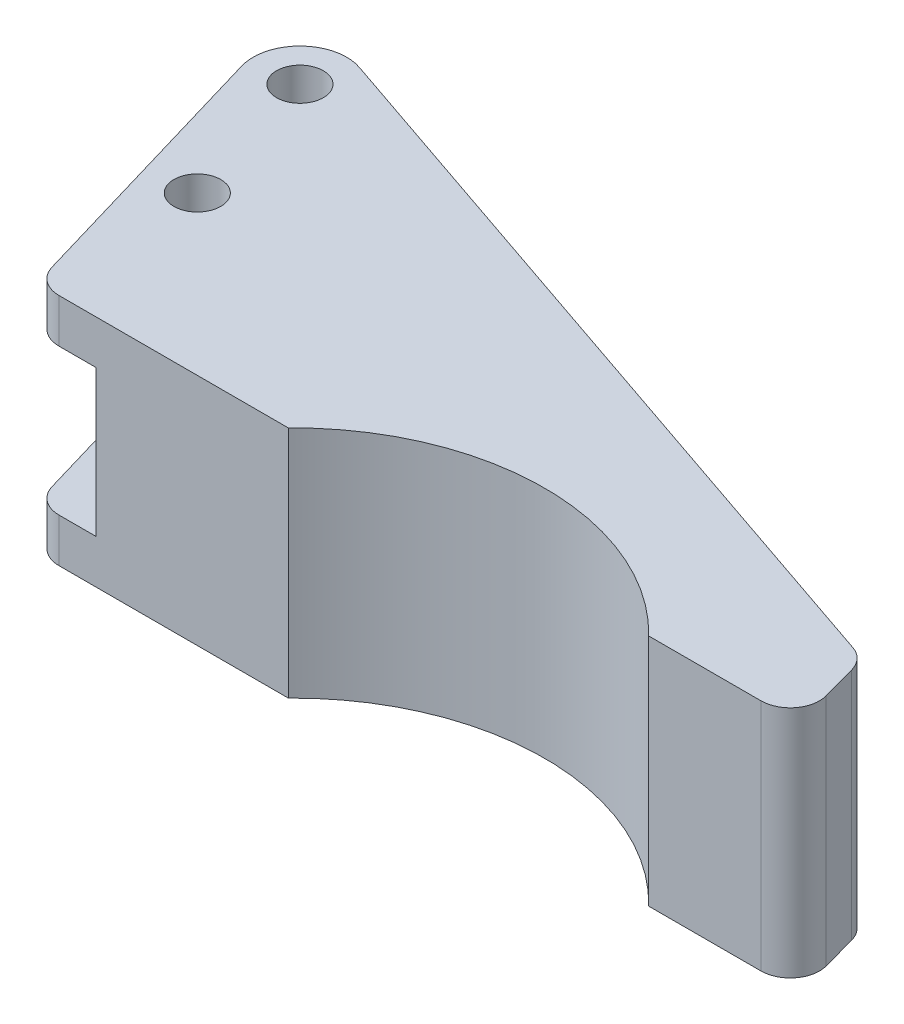
ISO-10303-21;
HEADER;
FILE_DESCRIPTION(('STEP AP214'),'2;1');
FILE_NAME('part.step','',(''),(''),'','','');
FILE_SCHEMA(('AUTOMOTIVE_DESIGN { 1 0 10303 214 1 1 1 1 }'));
ENDSEC;
DATA;
#1=APPLICATION_CONTEXT('core data for automotive mechanical design processes');
#2=APPLICATION_PROTOCOL_DEFINITION('international standard','automotive_design',2000,#1);
#3=PRODUCT_CONTEXT('',#1,'mechanical');
#4=PRODUCT('Part','Part','',(#3));
#5=PRODUCT_RELATED_PRODUCT_CATEGORY('part','',(#4));
#6=PRODUCT_DEFINITION_FORMATION('','',#4);
#7=PRODUCT_DEFINITION_CONTEXT('part definition',#1,'design');
#8=PRODUCT_DEFINITION('design','',#6,#7);
#9=PRODUCT_DEFINITION_SHAPE('','',#8);
#10=(LENGTH_UNIT() NAMED_UNIT(*) SI_UNIT(.MILLI.,.METRE.));
#11=(NAMED_UNIT(*) PLANE_ANGLE_UNIT() SI_UNIT($,.RADIAN.));
#12=(NAMED_UNIT(*) SI_UNIT($,.STERADIAN.) SOLID_ANGLE_UNIT());
#13=UNCERTAINTY_MEASURE_WITH_UNIT(LENGTH_MEASURE(1.E-05),#10,'distance_accuracy_value','');
#14=(GEOMETRIC_REPRESENTATION_CONTEXT(3) GLOBAL_UNCERTAINTY_ASSIGNED_CONTEXT((#13)) GLOBAL_UNIT_ASSIGNED_CONTEXT((#10,
#11,#12)) REPRESENTATION_CONTEXT('',''));
#15=CARTESIAN_POINT('',(0.,0.,0.));
#16=DIRECTION('',(0.,0.,1.));
#17=DIRECTION('',(1.,0.,0.));
#18=AXIS2_PLACEMENT_3D('',#15,#16,#17);
#19=CARTESIAN_POINT('',(-6.95128705790323,20.,-51.87));
#20=DIRECTION('',(0.,-1.,0.));
#21=DIRECTION('',(0.,0.,-1.));
#22=AXIS2_PLACEMENT_3D('',#19,#20,#21);
#23=CYLINDRICAL_SURFACE('',#22,8.);
#24=CARTESIAN_POINT('',(-6.95128705790323,12.5,-51.87));
#25=DIRECTION('',(0.,1.,0.));
#26=DIRECTION('',(0.,0.,1.));
#27=AXIS2_PLACEMENT_3D('',#24,#25,#26);
#28=CIRCLE('',#27,8.);
#29=CARTESIAN_POINT('',(-4.36732030928919,12.5,-59.4412030643787));
#30=VERTEX_POINT('',#29);
#31=CARTESIAN_POINT('',(-14.6247754698929,12.5,-49.607794087387));
#32=VERTEX_POINT('',#31);
#33=EDGE_CURVE('E247',#30,#32,#28,.T.);
#34=ORIENTED_EDGE('',*,*,#33,.T.);
#35=DIRECTION('',(0.,-1.,0.));
#36=VECTOR('',#35,1.);
#37=CARTESIAN_POINT('',(-14.6247754698928,20.,-49.607794087387));
#38=LINE('',#37,#36);
#39=CARTESIAN_POINT('',(-14.6247754698928,20.,-49.607794087387));
#40=VERTEX_POINT('',#39);
#41=EDGE_CURVE('E192',#40,#32,#38,.T.);
#42=ORIENTED_EDGE('',*,*,#41,.F.);
#43=CARTESIAN_POINT('',(-6.95128705790323,20.,-51.87));
#44=DIRECTION('',(0.,1.,0.));
#45=DIRECTION('',(0.,0.,1.));
#46=AXIS2_PLACEMENT_3D('',#43,#44,#45);
#47=CIRCLE('',#46,8.);
#48=CARTESIAN_POINT('',(-4.36732030928919,20.,-59.4412030643787));
#49=VERTEX_POINT('',#48);
#50=EDGE_CURVE('E143',#49,#40,#47,.T.);
#51=ORIENTED_EDGE('',*,*,#50,.F.);
#52=DIRECTION('',(0.,-1.,0.));
#53=VECTOR('',#52,1.);
#54=CARTESIAN_POINT('',(-4.36732030928919,20.,-59.4412030643787));
#55=LINE('',#54,#53);
#56=EDGE_CURVE('E196',#49,#30,#55,.T.);
#57=ORIENTED_EDGE('',*,*,#56,.T.);
#58=EDGE_LOOP('',(#34,#42,#51,#57));
#59=FACE_BOUND('',#58,.T.);
#60=ADVANCED_FACE('F41',(#59),#23,.T.);
#61=CARTESIAN_POINT('',(-1.05721731539673,20.,-3.5861213046169));
#62=DIRECTION('',(0.959186051498703,0.,-0.282775739076619));
#63=DIRECTION('',(-0.282775739076619,0.,-0.959186051498703));
#64=AXIS2_PLACEMENT_3D('',#61,#62,#63);
#65=PLANE('',#64);
#66=ORIENTED_EDGE('',*,*,#41,.T.);
#67=DIRECTION('',(0.282775739076619,0.,0.959186051498703));
#68=VECTOR('',#67,1.);
#69=CARTESIAN_POINT('',(-1.05721731539673,12.5,-3.5861213046169));
#70=LINE('',#69,#68);
#71=CARTESIAN_POINT('',(-1.05721731539673,12.5,-3.5861213046169));
#72=VERTEX_POINT('',#71);
#73=EDGE_CURVE('E155',#32,#72,#70,.T.);
#74=ORIENTED_EDGE('',*,*,#73,.T.);
#75=DIRECTION('',(0.,-1.,0.));
#76=VECTOR('',#75,1.);
#77=CARTESIAN_POINT('',(-1.05721731539673,20.,-3.5861213046169));
#78=LINE('',#77,#76);
#79=CARTESIAN_POINT('',(-1.05721731539673,20.,-3.5861213046169));
#80=VERTEX_POINT('',#79);
#81=EDGE_CURVE('E146',#80,#72,#78,.T.);
#82=ORIENTED_EDGE('',*,*,#81,.F.);
#83=DIRECTION('',(0.282775739076619,0.,0.959186051498703));
#84=VECTOR('',#83,1.);
#85=CARTESIAN_POINT('',(-1.05721731539673,20.,-3.5861213046169));
#86=LINE('',#85,#84);
#87=EDGE_CURVE('E135',#40,#80,#86,.T.);
#88=ORIENTED_EDGE('',*,*,#87,.F.);
#89=EDGE_LOOP('',(#66,#74,#82,#88));
#90=FACE_BOUND('',#89,.T.);
#91=ADVANCED_FACE('F149',(#90),#65,.F.);
#92=CARTESIAN_POINT('',(3.73871294209678,20.,-4.99999999999999));
#93=DIRECTION('',(0.,-1.,0.));
#94=DIRECTION('',(0.,0.,-1.));
#95=AXIS2_PLACEMENT_3D('',#92,#93,#94);
#96=CYLINDRICAL_SURFACE('',#95,5.);
#97=ORIENTED_EDGE('',*,*,#81,.T.);
#98=CARTESIAN_POINT('',(3.73871294209678,12.5,-4.99999999999999));
#99=DIRECTION('',(0.,1.,0.));
#100=DIRECTION('',(0.,0.,1.));
#101=AXIS2_PLACEMENT_3D('',#98,#99,#100);
#102=CIRCLE('',#101,5.);
#103=CARTESIAN_POINT('',(3.73871294209678,12.5,0.));
#104=VERTEX_POINT('',#103);
#105=EDGE_CURVE('E250',#72,#104,#102,.T.);
#106=ORIENTED_EDGE('',*,*,#105,.T.);
#107=DIRECTION('',(0.,-1.,0.));
#108=VECTOR('',#107,1.);
#109=CARTESIAN_POINT('',(3.73871294209678,20.,0.));
#110=LINE('',#109,#108);
#111=CARTESIAN_POINT('',(3.73871294209678,20.,0.));
#112=VERTEX_POINT('',#111);
#113=EDGE_CURVE('E159',#112,#104,#110,.T.);
#114=ORIENTED_EDGE('',*,*,#113,.F.);
#115=CARTESIAN_POINT('',(3.73871294209678,20.,-4.99999999999999));
#116=DIRECTION('',(0.,1.,0.));
#117=DIRECTION('',(0.,0.,1.));
#118=AXIS2_PLACEMENT_3D('',#115,#116,#117);
#119=CIRCLE('',#118,5.);
#120=EDGE_CURVE('E136',#80,#112,#119,.T.);
#121=ORIENTED_EDGE('',*,*,#120,.F.);
#122=EDGE_LOOP('',(#97,#106,#114,#121));
#123=FACE_BOUND('',#122,.T.);
#124=ADVANCED_FACE('F158',(#123),#96,.T.);
#125=CARTESIAN_POINT('',(0.378712942096768,-20.,-27.));
#126=DIRECTION('',(0.,1.,0.));
#127=DIRECTION('',(0.,0.,1.));
#128=AXIS2_PLACEMENT_3D('',#125,#126,#127);
#129=CYLINDRICAL_SURFACE('',#128,4.);
#130=CARTESIAN_POINT('',(0.378712942096768,12.5,-27.));
#131=DIRECTION('',(0.,1.,0.));
#132=DIRECTION('',(0.,0.,1.));
#133=AXIS2_PLACEMENT_3D('',#130,#131,#132);
#134=CIRCLE('',#133,4.);
#135=CARTESIAN_POINT('',(0.378712942096768,12.5,-23.));
#136=VERTEX_POINT('',#135);
#137=EDGE_CURVE('E245',#136,#136,#134,.F.);
#138=ORIENTED_EDGE('',*,*,#137,.T.);
#139=EDGE_LOOP('',(#138));
#140=FACE_BOUND('',#139,.T.);
#141=CARTESIAN_POINT('',(0.378712942096768,20.,-27.));
#142=DIRECTION('',(0.,1.,0.));
#143=DIRECTION('',(0.,0.,1.));
#144=AXIS2_PLACEMENT_3D('',#141,#142,#143);
#145=CIRCLE('',#144,4.);
#146=CARTESIAN_POINT('',(0.378712942096768,20.,-23.));
#147=VERTEX_POINT('',#146);
#148=EDGE_CURVE('E264',#147,#147,#145,.T.);
#149=ORIENTED_EDGE('',*,*,#148,.T.);
#150=EDGE_LOOP('',(#149));
#151=FACE_BOUND('',#150,.T.);
#152=ADVANCED_FACE('F362',(#140,#151),#129,.F.);
#153=CARTESIAN_POINT('',(-6.95128705790323,-20.,-51.87));
#154=DIRECTION('',(0.,1.,0.));
#155=DIRECTION('',(0.,0.,1.));
#156=AXIS2_PLACEMENT_3D('',#153,#154,#155);
#157=CYLINDRICAL_SURFACE('',#156,4.);
#158=CARTESIAN_POINT('',(-6.95128705790323,12.5,-51.87));
#159=DIRECTION('',(0.,1.,0.));
#160=DIRECTION('',(0.,0.,1.));
#161=AXIS2_PLACEMENT_3D('',#158,#159,#160);
#162=CIRCLE('',#161,4.);
#163=CARTESIAN_POINT('',(-6.95128705790323,12.5,-47.87));
#164=VERTEX_POINT('',#163);
#165=EDGE_CURVE('E44',#164,#164,#162,.F.);
#166=ORIENTED_EDGE('',*,*,#165,.T.);
#167=EDGE_LOOP('',(#166));
#168=FACE_BOUND('',#167,.T.);
#169=CARTESIAN_POINT('',(-6.95128705790323,20.,-51.87));
#170=DIRECTION('',(0.,1.,0.));
#171=DIRECTION('',(0.,0.,1.));
#172=AXIS2_PLACEMENT_3D('',#169,#170,#171);
#173=CIRCLE('',#172,4.);
#174=CARTESIAN_POINT('',(-6.95128705790323,20.,-47.87));
#175=VERTEX_POINT('',#174);
#176=EDGE_CURVE('E265',#175,#175,#173,.T.);
#177=ORIENTED_EDGE('',*,*,#176,.T.);
#178=EDGE_LOOP('',(#177));
#179=FACE_BOUND('',#178,.T.);
#180=ADVANCED_FACE('F390',(#168,#179),#157,.F.);
#181=CARTESIAN_POINT('',(73.7387129420968,20.,30.));
#182=DIRECTION('',(0.,-1.,0.));
#183=DIRECTION('',(0.,0.,-1.));
#184=AXIS2_PLACEMENT_3D('',#181,#182,#183);
#185=CYLINDRICAL_SURFACE('',#184,43.);
#186=CARTESIAN_POINT('',(73.7387129420968,-20.,30.));
#187=DIRECTION('',(0.,-1.,0.));
#188=DIRECTION('',(0.,0.,1.));
#189=AXIS2_PLACEMENT_3D('',#186,#187,#188);
#190=CIRCLE('',#189,43.);
#191=CARTESIAN_POINT('',(42.9328693405981,-20.,0.));
#192=VERTEX_POINT('',#191);
#193=CARTESIAN_POINT('',(104.544556543596,-20.,0.));
#194=VERTEX_POINT('',#193);
#195=EDGE_CURVE('E167',#192,#194,#190,.T.);
#196=ORIENTED_EDGE('',*,*,#195,.T.);
#197=DIRECTION('',(0.,-1.,0.));
#198=VECTOR('',#197,1.);
#199=CARTESIAN_POINT('',(104.544556543596,20.,0.));
#200=LINE('',#199,#198);
#201=CARTESIAN_POINT('',(104.544556543596,20.,0.));
#202=VERTEX_POINT('',#201);
#203=EDGE_CURVE('E11',#202,#194,#200,.T.);
#204=ORIENTED_EDGE('',*,*,#203,.F.);
#205=CARTESIAN_POINT('',(73.7387129420968,20.,30.));
#206=DIRECTION('',(0.,-1.,0.));
#207=DIRECTION('',(0.,0.,1.));
#208=AXIS2_PLACEMENT_3D('',#205,#206,#207);
#209=CIRCLE('',#208,43.);
#210=CARTESIAN_POINT('',(42.9328693405981,20.,0.));
#211=VERTEX_POINT('',#210);
#212=EDGE_CURVE('E193',#211,#202,#209,.T.);
#213=ORIENTED_EDGE('',*,*,#212,.F.);
#214=DIRECTION('',(0.,-1.,0.));
#215=VECTOR('',#214,1.);
#216=CARTESIAN_POINT('',(42.9328693405981,20.,0.));
#217=LINE('',#216,#215);
#218=EDGE_CURVE('E165',#211,#192,#217,.T.);
#219=ORIENTED_EDGE('',*,*,#218,.T.);
#220=EDGE_LOOP('',(#196,#204,#213,#219));
#221=FACE_BOUND('',#220,.T.);
#222=ADVANCED_FACE('F43',(#221),#185,.F.);
#223=CARTESIAN_POINT('',(123.738712942097,20.,0.));
#224=DIRECTION('',(0.,0.,-1.));
#225=DIRECTION('',(-1.,0.,0.));
#226=AXIS2_PLACEMENT_3D('',#223,#224,#225);
#227=PLANE('',#226);
#228=DIRECTION('',(1.,0.,0.));
#229=VECTOR('',#228,1.);
#230=CARTESIAN_POINT('',(123.738712942097,-20.,0.));
#231=LINE('',#230,#229);
#232=CARTESIAN_POINT('',(123.738712942097,-20.,0.));
#233=VERTEX_POINT('',#232);
#234=EDGE_CURVE('E166',#194,#233,#231,.T.);
#235=ORIENTED_EDGE('',*,*,#234,.T.);
#236=DIRECTION('',(0.,-1.,0.));
#237=VECTOR('',#236,1.);
#238=CARTESIAN_POINT('',(123.738712942097,20.,0.));
#239=LINE('',#238,#237);
#240=CARTESIAN_POINT('',(123.738712942097,20.,0.));
#241=VERTEX_POINT('',#240);
#242=EDGE_CURVE('E49',#241,#233,#239,.T.);
#243=ORIENTED_EDGE('',*,*,#242,.F.);
#244=DIRECTION('',(1.,0.,0.));
#245=VECTOR('',#244,1.);
#246=CARTESIAN_POINT('',(123.738712942097,20.,0.));
#247=LINE('',#246,#245);
#248=EDGE_CURVE('E114',#202,#241,#247,.T.);
#249=ORIENTED_EDGE('',*,*,#248,.F.);
#250=ORIENTED_EDGE('',*,*,#203,.T.);
#251=EDGE_LOOP('',(#235,#243,#249,#250));
#252=FACE_BOUND('',#251,.T.);
#253=ADVANCED_FACE('F326',(#252),#227,.F.);
#254=CARTESIAN_POINT('',(123.738712942097,20.,-5.));
#255=DIRECTION('',(0.,-1.,0.));
#256=DIRECTION('',(0.,0.,-1.));
#257=AXIS2_PLACEMENT_3D('',#254,#255,#256);
#258=CYLINDRICAL_SURFACE('',#257,4.99999999999999);
#259=CARTESIAN_POINT('',(123.738712942097,-20.,-5.));
#260=DIRECTION('',(0.,1.,0.));
#261=DIRECTION('',(0.,0.,-1.));
#262=AXIS2_PLACEMENT_3D('',#259,#260,#261);
#263=CIRCLE('',#262,4.99999999999999);
#264=CARTESIAN_POINT('',(128.559739906116,-20.,-6.32578241510522));
#265=VERTEX_POINT('',#264);
#266=EDGE_CURVE('E174',#233,#265,#263,.T.);
#267=ORIENTED_EDGE('',*,*,#266,.T.);
#268=DIRECTION('',(0.,-1.,0.));
#269=VECTOR('',#268,1.);
#270=CARTESIAN_POINT('',(128.559739906116,20.,-6.32578241510522));
#271=LINE('',#270,#269);
#272=CARTESIAN_POINT('',(128.559739906116,20.,-6.32578241510522));
#273=VERTEX_POINT('',#272);
#274=EDGE_CURVE('E210',#273,#265,#271,.T.);
#275=ORIENTED_EDGE('',*,*,#274,.F.);
#276=CARTESIAN_POINT('',(123.738712942097,20.,-5.));
#277=DIRECTION('',(0.,1.,0.));
#278=DIRECTION('',(0.,0.,-1.));
#279=AXIS2_PLACEMENT_3D('',#276,#277,#278);
#280=CIRCLE('',#279,4.99999999999999);
#281=EDGE_CURVE('E275',#241,#273,#280,.T.);
#282=ORIENTED_EDGE('',*,*,#281,.F.);
#283=ORIENTED_EDGE('',*,*,#242,.T.);
#284=EDGE_LOOP('',(#267,#275,#282,#283));
#285=FACE_BOUND('',#284,.T.);
#286=ADVANCED_FACE('F328',(#285),#258,.T.);
#287=CARTESIAN_POINT('',(126.909739906116,20.,-12.3257824151052));
#288=DIRECTION('',(-0.964205392803791,0.,0.26515648302104));
#289=DIRECTION('',(0.26515648302104,0.,0.964205392803791));
#290=AXIS2_PLACEMENT_3D('',#287,#288,#289);
#291=PLANE('',#290);
#292=DIRECTION('',(-0.26515648302104,0.,-0.964205392803791));
#293=VECTOR('',#292,1.);
#294=CARTESIAN_POINT('',(126.909739906116,-20.,-12.3257824151052));
#295=LINE('',#294,#293);
#296=CARTESIAN_POINT('',(126.909739906116,-20.,-12.3257824151052));
#297=VERTEX_POINT('',#296);
#298=EDGE_CURVE('E175',#265,#297,#295,.T.);
#299=ORIENTED_EDGE('',*,*,#298,.T.);
#300=DIRECTION('',(0.,-1.,0.));
#301=VECTOR('',#300,1.);
#302=CARTESIAN_POINT('',(126.909739906116,20.,-12.3257824151052));
#303=LINE('',#302,#301);
#304=CARTESIAN_POINT('',(126.909739906116,20.,-12.3257824151052));
#305=VERTEX_POINT('',#304);
#306=EDGE_CURVE('E204',#305,#297,#303,.T.);
#307=ORIENTED_EDGE('',*,*,#306,.F.);
#308=DIRECTION('',(-0.26515648302104,0.,-0.964205392803791));
#309=VECTOR('',#308,1.);
#310=CARTESIAN_POINT('',(126.909739906116,20.,-12.3257824151052));
#311=LINE('',#310,#309);
#312=EDGE_CURVE('E273',#273,#305,#311,.T.);
#313=ORIENTED_EDGE('',*,*,#312,.F.);
#314=ORIENTED_EDGE('',*,*,#274,.T.);
#315=EDGE_LOOP('',(#299,#307,#313,#314));
#316=FACE_BOUND('',#315,.T.);
#317=ADVANCED_FACE('F331',(#316),#291,.F.);
#318=CARTESIAN_POINT('',(122.088712942097,20.,-11.));
#319=DIRECTION('',(0.,-1.,0.));
#320=DIRECTION('',(0.,0.,-1.));
#321=AXIS2_PLACEMENT_3D('',#318,#319,#320);
#322=CYLINDRICAL_SURFACE('',#321,5.00000000000001);
#323=CARTESIAN_POINT('',(122.088712942097,-20.,-11.));
#324=DIRECTION('',(0.,1.,0.));
#325=DIRECTION('',(0.,0.,1.));
#326=AXIS2_PLACEMENT_3D('',#323,#324,#325);
#327=CIRCLE('',#326,5.00000000000001);
#328=CARTESIAN_POINT('',(123.703692159981,-20.,-15.7320019152367));
#329=VERTEX_POINT('',#328);
#330=EDGE_CURVE('E178',#297,#329,#327,.T.);
#331=ORIENTED_EDGE('',*,*,#330,.T.);
#332=DIRECTION('',(0.,-1.,0.));
#333=VECTOR('',#332,1.);
#334=CARTESIAN_POINT('',(123.703692159981,20.,-15.7320019152367));
#335=LINE('',#334,#333);
#336=CARTESIAN_POINT('',(123.703692159981,20.,-15.7320019152367));
#337=VERTEX_POINT('',#336);
#338=EDGE_CURVE('E203',#337,#329,#335,.T.);
#339=ORIENTED_EDGE('',*,*,#338,.F.);
#340=CARTESIAN_POINT('',(122.088712942097,20.,-11.));
#341=DIRECTION('',(0.,1.,0.));
#342=DIRECTION('',(0.,0.,1.));
#343=AXIS2_PLACEMENT_3D('',#340,#341,#342);
#344=CIRCLE('',#343,5.00000000000001);
#345=EDGE_CURVE('E277',#305,#337,#344,.T.);
#346=ORIENTED_EDGE('',*,*,#345,.F.);
#347=ORIENTED_EDGE('',*,*,#306,.T.);
#348=EDGE_LOOP('',(#331,#339,#346,#347));
#349=FACE_BOUND('',#348,.T.);
#350=ADVANCED_FACE('F339',(#349),#322,.T.);
#351=CARTESIAN_POINT('',(-4.36732030928919,20.,-59.4412030643787));
#352=DIRECTION('',(-0.322995843576755,0.,0.946400383047334));
#353=DIRECTION('',(0.946400383047334,0.,0.322995843576755));
#354=AXIS2_PLACEMENT_3D('',#351,#352,#353);
#355=PLANE('',#354);
#356=DIRECTION('',(0.,1.,0.));
#357=VECTOR('',#356,1.);
#358=CARTESIAN_POINT('',(10.0487129420968,20.,-54.5211724890856));
#359=LINE('',#358,#357);
#360=CARTESIAN_POINT('',(10.0487129420968,-12.5,-54.5211724890856));
#361=VERTEX_POINT('',#360);
#362=CARTESIAN_POINT('',(10.0487129420968,12.5,-54.5211724890856));
#363=VERTEX_POINT('',#362);
#364=EDGE_CURVE('E258',#361,#363,#359,.T.);
#365=ORIENTED_EDGE('',*,*,#364,.T.);
#366=DIRECTION('',(-0.946400383047334,0.,-0.322995843576755));
#367=VECTOR('',#366,1.);
#368=CARTESIAN_POINT('',(-4.36732030928919,12.5,-59.4412030643787));
#369=LINE('',#368,#367);
#370=EDGE_CURVE('E251',#363,#30,#369,.T.);
#371=ORIENTED_EDGE('',*,*,#370,.T.);
#372=ORIENTED_EDGE('',*,*,#56,.F.);
#373=DIRECTION('',(-0.946400383047334,0.,-0.322995843576755));
#374=VECTOR('',#373,1.);
#375=CARTESIAN_POINT('',(-4.36732030928919,20.,-59.4412030643787));
#376=LINE('',#375,#374);
#377=EDGE_CURVE('E279',#337,#49,#376,.T.);
#378=ORIENTED_EDGE('',*,*,#377,.F.);
#379=ORIENTED_EDGE('',*,*,#338,.T.);
#380=DIRECTION('',(-0.946400383047334,0.,-0.322995843576755));
#381=VECTOR('',#380,1.);
#382=CARTESIAN_POINT('',(-4.36732030928919,-20.,-59.4412030643787));
#383=LINE('',#382,#381);
#384=CARTESIAN_POINT('',(-4.36732030928919,-20.,-59.4412030643787));
#385=VERTEX_POINT('',#384);
#386=EDGE_CURVE('E176',#329,#385,#383,.T.);
#387=ORIENTED_EDGE('',*,*,#386,.T.);
#388=CARTESIAN_POINT('',(-4.36732030928919,-12.5,-59.4412030643787));
#389=VERTEX_POINT('',#388);
#390=EDGE_CURVE('E197',#389,#385,#55,.T.);
#391=ORIENTED_EDGE('',*,*,#390,.F.);
#392=DIRECTION('',(0.946400383047334,0.,0.322995843576755));
#393=VECTOR('',#392,1.);
#394=CARTESIAN_POINT('',(-4.36732030928919,-12.5,-59.4412030643787));
#395=LINE('',#394,#393);
#396=EDGE_CURVE('E243',#389,#361,#395,.T.);
#397=ORIENTED_EDGE('',*,*,#396,.T.);
#398=EDGE_LOOP('',(#365,#371,#372,#378,#379,#387,#391,#397));
#399=FACE_BOUND('',#398,.T.);
#400=ADVANCED_FACE('F285',(#399),#355,.F.);
#401=CARTESIAN_POINT('',(-14.6247754698929,-12.5,-49.607794087387));
#402=VERTEX_POINT('',#401);
#403=CARTESIAN_POINT('',(-14.6247754698928,-20.,-49.607794087387));
#404=VERTEX_POINT('',#403);
#405=EDGE_CURVE('E154',#402,#404,#38,.T.);
#406=ORIENTED_EDGE('',*,*,#405,.F.);
#407=CARTESIAN_POINT('',(-6.95128705790323,-12.5,-51.87));
#408=DIRECTION('',(0.,-1.,0.));
#409=DIRECTION('',(1.,0.,0.));
#410=AXIS2_PLACEMENT_3D('',#407,#408,#409);
#411=CIRCLE('',#410,8.);
#412=EDGE_CURVE('E236',#402,#389,#411,.T.);
#413=ORIENTED_EDGE('',*,*,#412,.T.);
#414=ORIENTED_EDGE('',*,*,#390,.T.);
#415=CARTESIAN_POINT('',(-6.95128705790323,-20.,-51.87));
#416=DIRECTION('',(0.,1.,0.));
#417=DIRECTION('',(0.,0.,1.));
#418=AXIS2_PLACEMENT_3D('',#415,#416,#417);
#419=CIRCLE('',#418,8.);
#420=EDGE_CURVE('E182',#385,#404,#419,.T.);
#421=ORIENTED_EDGE('',*,*,#420,.T.);
#422=EDGE_LOOP('',(#406,#413,#414,#421));
#423=FACE_BOUND('',#422,.T.);
#424=ADVANCED_FACE('F350',(#423),#23,.T.);
#425=CARTESIAN_POINT('',(-1.05721731539673,-12.5,-3.5861213046169));
#426=VERTEX_POINT('',#425);
#427=CARTESIAN_POINT('',(-1.05721731539673,-20.,-3.5861213046169));
#428=VERTEX_POINT('',#427);
#429=EDGE_CURVE('E156',#426,#428,#78,.T.);
#430=ORIENTED_EDGE('',*,*,#429,.F.);
#431=DIRECTION('',(-0.282775739076619,0.,-0.959186051498703));
#432=VECTOR('',#431,1.);
#433=CARTESIAN_POINT('',(-1.05721731539673,-12.5,-3.5861213046169));
#434=LINE('',#433,#432);
#435=EDGE_CURVE('E232',#426,#402,#434,.T.);
#436=ORIENTED_EDGE('',*,*,#435,.T.);
#437=ORIENTED_EDGE('',*,*,#405,.T.);
#438=DIRECTION('',(0.282775739076619,0.,0.959186051498703));
#439=VECTOR('',#438,1.);
#440=CARTESIAN_POINT('',(-1.05721731539673,-20.,-3.5861213046169));
#441=LINE('',#440,#439);
#442=EDGE_CURVE('E184',#404,#428,#441,.T.);
#443=ORIENTED_EDGE('',*,*,#442,.T.);
#444=EDGE_LOOP('',(#430,#436,#437,#443));
#445=FACE_BOUND('',#444,.T.);
#446=ADVANCED_FACE('F348',(#445),#65,.F.);
#447=CARTESIAN_POINT('',(3.73871294209678,-12.5,0.));
#448=VERTEX_POINT('',#447);
#449=CARTESIAN_POINT('',(3.73871294209678,-20.,0.));
#450=VERTEX_POINT('',#449);
#451=EDGE_CURVE('E191',#448,#450,#110,.T.);
#452=ORIENTED_EDGE('',*,*,#451,.F.);
#453=CARTESIAN_POINT('',(3.73871294209678,-12.5,-4.99999999999999));
#454=DIRECTION('',(0.,-1.,0.));
#455=DIRECTION('',(1.,0.,0.));
#456=AXIS2_PLACEMENT_3D('',#453,#454,#455);
#457=CIRCLE('',#456,5.);
#458=EDGE_CURVE('E59',#448,#426,#457,.T.);
#459=ORIENTED_EDGE('',*,*,#458,.T.);
#460=ORIENTED_EDGE('',*,*,#429,.T.);
#461=CARTESIAN_POINT('',(3.73871294209678,-20.,-4.99999999999999));
#462=DIRECTION('',(0.,1.,0.));
#463=DIRECTION('',(0.,0.,1.));
#464=AXIS2_PLACEMENT_3D('',#461,#462,#463);
#465=CIRCLE('',#464,5.);
#466=EDGE_CURVE('E189',#428,#450,#465,.T.);
#467=ORIENTED_EDGE('',*,*,#466,.T.);
#468=EDGE_LOOP('',(#452,#459,#460,#467));
#469=FACE_BOUND('',#468,.T.);
#470=ADVANCED_FACE('F354',(#469),#96,.T.);
#471=CARTESIAN_POINT('',(42.9328693405981,20.,0.));
#472=DIRECTION('',(0.,0.,-1.));
#473=DIRECTION('',(-1.,0.,0.));
#474=AXIS2_PLACEMENT_3D('',#471,#472,#473);
#475=PLANE('',#474);
#476=ORIENTED_EDGE('',*,*,#113,.T.);
#477=DIRECTION('',(-1.,0.,0.));
#478=VECTOR('',#477,1.);
#479=CARTESIAN_POINT('',(-14.9512870579032,12.5,0.));
#480=LINE('',#479,#478);
#481=CARTESIAN_POINT('',(10.0487129420968,12.5,0.));
#482=VERTEX_POINT('',#481);
#483=EDGE_CURVE('E230',#482,#104,#480,.T.);
#484=ORIENTED_EDGE('',*,*,#483,.F.);
#485=DIRECTION('',(0.,1.,0.));
#486=VECTOR('',#485,1.);
#487=CARTESIAN_POINT('',(10.0487129420968,12.5,0.));
#488=LINE('',#487,#486);
#489=CARTESIAN_POINT('',(10.0487129420968,-12.5,0.));
#490=VERTEX_POINT('',#489);
#491=EDGE_CURVE('E315',#490,#482,#488,.T.);
#492=ORIENTED_EDGE('',*,*,#491,.F.);
#493=DIRECTION('',(1.,0.,0.));
#494=VECTOR('',#493,1.);
#495=CARTESIAN_POINT('',(-14.9512870579032,-12.5,0.));
#496=LINE('',#495,#494);
#497=EDGE_CURVE('E314',#448,#490,#496,.T.);
#498=ORIENTED_EDGE('',*,*,#497,.F.);
#499=ORIENTED_EDGE('',*,*,#451,.T.);
#500=DIRECTION('',(1.,0.,0.));
#501=VECTOR('',#500,1.);
#502=CARTESIAN_POINT('',(42.9328693405981,-20.,0.));
#503=LINE('',#502,#501);
#504=EDGE_CURVE('E104',#450,#192,#503,.T.);
#505=ORIENTED_EDGE('',*,*,#504,.T.);
#506=ORIENTED_EDGE('',*,*,#218,.F.);
#507=DIRECTION('',(1.,0.,0.));
#508=VECTOR('',#507,1.);
#509=CARTESIAN_POINT('',(42.9328693405981,20.,0.));
#510=LINE('',#509,#508);
#511=EDGE_CURVE('E70',#112,#211,#510,.T.);
#512=ORIENTED_EDGE('',*,*,#511,.F.);
#513=EDGE_LOOP('',(#476,#484,#492,#498,#499,#505,#506,#512));
#514=FACE_BOUND('',#513,.T.);
#515=ADVANCED_FACE('F318',(#514),#475,.F.);
#516=CARTESIAN_POINT('',(73.7387129420968,20.,30.));
#517=DIRECTION('',(0.,1.,0.));
#518=DIRECTION('',(0.,0.,1.));
#519=AXIS2_PLACEMENT_3D('',#516,#517,#518);
#520=PLANE('',#519);
#521=ORIENTED_EDGE('',*,*,#176,.F.);
#522=EDGE_LOOP('',(#521));
#523=FACE_BOUND('',#522,.T.);
#524=ORIENTED_EDGE('',*,*,#148,.F.);
#525=EDGE_LOOP('',(#524));
#526=FACE_BOUND('',#525,.T.);
#527=ORIENTED_EDGE('',*,*,#212,.T.);
#528=ORIENTED_EDGE('',*,*,#248,.T.);
#529=ORIENTED_EDGE('',*,*,#281,.T.);
#530=ORIENTED_EDGE('',*,*,#312,.T.);
#531=ORIENTED_EDGE('',*,*,#345,.T.);
#532=ORIENTED_EDGE('',*,*,#377,.T.);
#533=ORIENTED_EDGE('',*,*,#50,.T.);
#534=ORIENTED_EDGE('',*,*,#87,.T.);
#535=ORIENTED_EDGE('',*,*,#120,.T.);
#536=ORIENTED_EDGE('',*,*,#511,.T.);
#537=EDGE_LOOP('',(#527,#528,#529,#530,#531,#532,#533,#534,#535,#536));
#538=FACE_BOUND('',#537,.T.);
#539=ADVANCED_FACE('F138',(#523,#526,#538),#520,.T.);
#540=CARTESIAN_POINT('',(73.7387129420968,-20.,30.));
#541=DIRECTION('',(0.,1.,0.));
#542=DIRECTION('',(0.,0.,1.));
#543=AXIS2_PLACEMENT_3D('',#540,#541,#542);
#544=PLANE('',#543);
#545=CARTESIAN_POINT('',(-6.95128705790323,-20.,-51.87));
#546=DIRECTION('',(0.,1.,0.));
#547=DIRECTION('',(0.,0.,1.));
#548=AXIS2_PLACEMENT_3D('',#545,#546,#547);
#549=CIRCLE('',#548,4.);
#550=CARTESIAN_POINT('',(-6.95128705790323,-20.,-47.87));
#551=VERTEX_POINT('',#550);
#552=EDGE_CURVE('E168',#551,#551,#549,.T.);
#553=ORIENTED_EDGE('',*,*,#552,.T.);
#554=EDGE_LOOP('',(#553));
#555=FACE_BOUND('',#554,.T.);
#556=CARTESIAN_POINT('',(0.378712942096768,-20.,-27.));
#557=DIRECTION('',(0.,1.,0.));
#558=DIRECTION('',(0.,0.,1.));
#559=AXIS2_PLACEMENT_3D('',#556,#557,#558);
#560=CIRCLE('',#559,4.);
#561=CARTESIAN_POINT('',(0.378712942096768,-20.,-23.));
#562=VERTEX_POINT('',#561);
#563=EDGE_CURVE('E259',#562,#562,#560,.T.);
#564=ORIENTED_EDGE('',*,*,#563,.T.);
#565=EDGE_LOOP('',(#564));
#566=FACE_BOUND('',#565,.T.);
#567=ORIENTED_EDGE('',*,*,#195,.F.);
#568=ORIENTED_EDGE('',*,*,#504,.F.);
#569=ORIENTED_EDGE('',*,*,#466,.F.);
#570=ORIENTED_EDGE('',*,*,#442,.F.);
#571=ORIENTED_EDGE('',*,*,#420,.F.);
#572=ORIENTED_EDGE('',*,*,#386,.F.);
#573=ORIENTED_EDGE('',*,*,#330,.F.);
#574=ORIENTED_EDGE('',*,*,#298,.F.);
#575=ORIENTED_EDGE('',*,*,#266,.F.);
#576=ORIENTED_EDGE('',*,*,#234,.F.);
#577=EDGE_LOOP('',(#567,#568,#569,#570,#571,#572,#573,#574,#575,#576));
#578=FACE_BOUND('',#577,.T.);
#579=ADVANCED_FACE('F345',(#555,#566,#578),#544,.F.);
#580=CARTESIAN_POINT('',(0.378712942096768,-12.5,-27.));
#581=DIRECTION('',(0.,-1.,0.));
#582=DIRECTION('',(1.,0.,0.));
#583=AXIS2_PLACEMENT_3D('',#580,#581,#582);
#584=CIRCLE('',#583,4.);
#585=CARTESIAN_POINT('',(4.37871294209677,-12.5,-27.));
#586=VERTEX_POINT('',#585);
#587=EDGE_CURVE('E213',#586,#586,#584,.F.);
#588=ORIENTED_EDGE('',*,*,#587,.T.);
#589=EDGE_LOOP('',(#588));
#590=FACE_BOUND('',#589,.T.);
#591=ORIENTED_EDGE('',*,*,#563,.F.);
#592=EDGE_LOOP('',(#591));
#593=FACE_BOUND('',#592,.T.);
#594=ADVANCED_FACE('F396',(#590,#593),#129,.F.);
#595=CARTESIAN_POINT('',(-6.95128705790323,-12.5,-51.87));
#596=DIRECTION('',(0.,-1.,0.));
#597=DIRECTION('',(1.,0.,0.));
#598=AXIS2_PLACEMENT_3D('',#595,#596,#597);
#599=CIRCLE('',#598,4.);
#600=CARTESIAN_POINT('',(-2.95128705790323,-12.5,-51.87));
#601=VERTEX_POINT('',#600);
#602=EDGE_CURVE('E211',#601,#601,#599,.F.);
#603=ORIENTED_EDGE('',*,*,#602,.T.);
#604=EDGE_LOOP('',(#603));
#605=FACE_BOUND('',#604,.T.);
#606=ORIENTED_EDGE('',*,*,#552,.F.);
#607=EDGE_LOOP('',(#606));
#608=FACE_BOUND('',#607,.T.);
#609=ADVANCED_FACE('F394',(#605,#608),#157,.F.);
#610=CARTESIAN_POINT('',(10.0487129420968,12.5,-59.87));
#611=DIRECTION('',(1.,0.,0.));
#612=DIRECTION('',(0.,1.,0.));
#613=AXIS2_PLACEMENT_3D('',#610,#611,#612);
#614=PLANE('',#613);
#615=DIRECTION('',(0.,0.,1.));
#616=VECTOR('',#615,1.);
#617=CARTESIAN_POINT('',(10.0487129420968,-12.5,-59.87));
#618=LINE('',#617,#616);
#619=EDGE_CURVE('E219',#361,#490,#618,.T.);
#620=ORIENTED_EDGE('',*,*,#619,.T.);
#621=ORIENTED_EDGE('',*,*,#491,.T.);
#622=DIRECTION('',(0.,0.,1.));
#623=VECTOR('',#622,1.);
#624=CARTESIAN_POINT('',(10.0487129420968,12.5,-59.87));
#625=LINE('',#624,#623);
#626=EDGE_CURVE('E212',#363,#482,#625,.T.);
#627=ORIENTED_EDGE('',*,*,#626,.F.);
#628=ORIENTED_EDGE('',*,*,#364,.F.);
#629=EDGE_LOOP('',(#620,#621,#627,#628));
#630=FACE_BOUND('',#629,.T.);
#631=ADVANCED_FACE('F309',(#630),#614,.F.);
#632=CARTESIAN_POINT('',(-14.9512870579032,12.5,-59.87));
#633=DIRECTION('',(0.,1.,0.));
#634=DIRECTION('',(0.,0.,1.));
#635=AXIS2_PLACEMENT_3D('',#632,#633,#634);
#636=PLANE('',#635);
#637=ORIENTED_EDGE('',*,*,#165,.F.);
#638=EDGE_LOOP('',(#637));
#639=FACE_BOUND('',#638,.T.);
#640=ORIENTED_EDGE('',*,*,#137,.F.);
#641=EDGE_LOOP('',(#640));
#642=FACE_BOUND('',#641,.T.);
#643=ORIENTED_EDGE('',*,*,#626,.T.);
#644=ORIENTED_EDGE('',*,*,#483,.T.);
#645=ORIENTED_EDGE('',*,*,#105,.F.);
#646=ORIENTED_EDGE('',*,*,#73,.F.);
#647=ORIENTED_EDGE('',*,*,#33,.F.);
#648=ORIENTED_EDGE('',*,*,#370,.F.);
#649=EDGE_LOOP('',(#643,#644,#645,#646,#647,#648));
#650=FACE_BOUND('',#649,.T.);
#651=ADVANCED_FACE('F317',(#639,#642,#650),#636,.F.);
#652=CARTESIAN_POINT('',(-14.9512870579032,-12.5,-59.87));
#653=DIRECTION('',(0.,-1.,0.));
#654=DIRECTION('',(1.,0.,0.));
#655=AXIS2_PLACEMENT_3D('',#652,#653,#654);
#656=PLANE('',#655);
#657=ORIENTED_EDGE('',*,*,#602,.F.);
#658=EDGE_LOOP('',(#657));
#659=FACE_BOUND('',#658,.T.);
#660=ORIENTED_EDGE('',*,*,#587,.F.);
#661=EDGE_LOOP('',(#660));
#662=FACE_BOUND('',#661,.T.);
#663=ORIENTED_EDGE('',*,*,#412,.F.);
#664=ORIENTED_EDGE('',*,*,#435,.F.);
#665=ORIENTED_EDGE('',*,*,#458,.F.);
#666=ORIENTED_EDGE('',*,*,#497,.T.);
#667=ORIENTED_EDGE('',*,*,#619,.F.);
#668=ORIENTED_EDGE('',*,*,#396,.F.);
#669=EDGE_LOOP('',(#663,#664,#665,#666,#667,#668));
#670=FACE_BOUND('',#669,.T.);
#671=ADVANCED_FACE('F312',(#659,#662,#670),#656,.F.);
#672=CLOSED_SHELL('',(#60,#91,#124,#152,#180,#222,#253,#286,#317,#350,#400,#424,#446,#470,#515,
#539,#579,#594,#609,#631,#651,#671));
#673=MANIFOLD_SOLID_BREP('B2',#672);
#674=ADVANCED_BREP_SHAPE_REPRESENTATION('',(#18,#673),#14);
#675=SHAPE_DEFINITION_REPRESENTATION(#9,#674);
ENDSEC;
END-ISO-10303-21;
